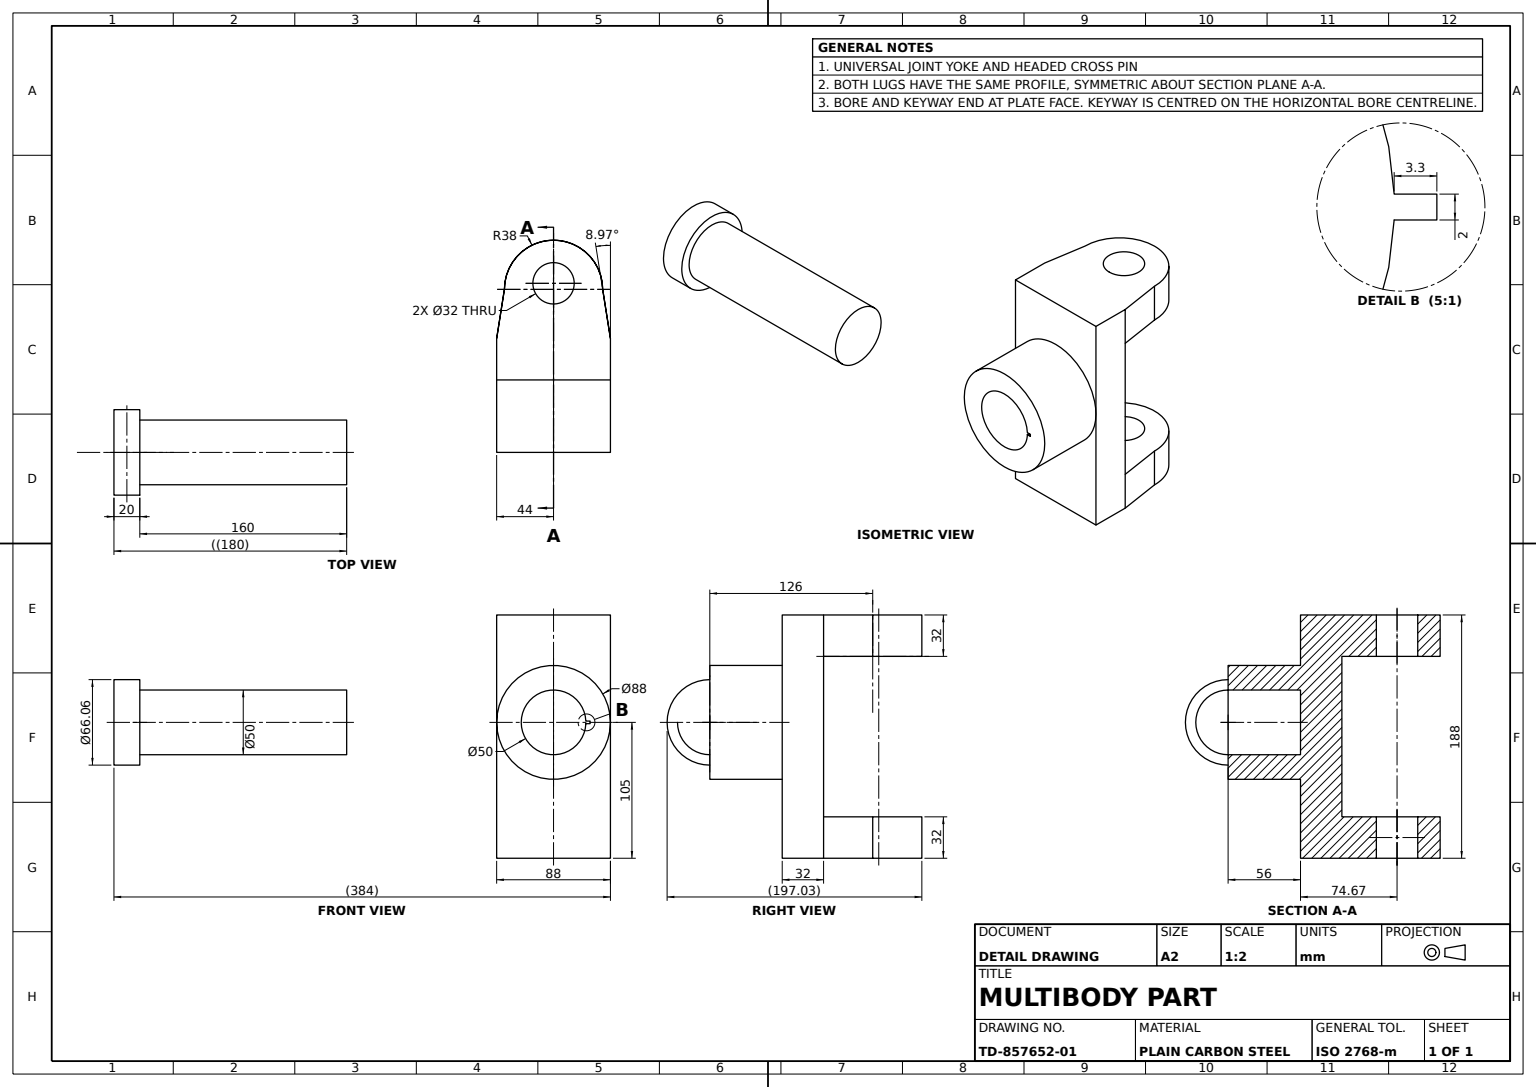
SolidWorks part; units mm, degrees
material "Plain Carbon Steel"
ref_plane "Front Plane" through (0, 0, 0) normal (0, 0, 1) x (1, 0, 0)
ref_plane "Top Plane" through (0, 0, 0) normal (0, 1, 0) x (1, 0, 0)
ref_plane "Right Plane" through (0, 0, 0) normal (1, 0, 0) x (0, 0, -1)
sketch "Hub Profile Ø88" plane through (0, 0, 0) normal (0, 0, 1) x (1, 0, 0)
  circle A0 centre (0, 0) radius 44
  dimension "D1" = 88
extrude "Hub Boss Ø88" add sketch "Hub Profile Ø88" along normal blind 56
sketch "Hub Cut Profile" plane through (0, 0, 0) normal (0, 0, -1) x (-1, 0, 0)
  line L1 (24.98, -0.9998) -> (24.98, -1.0002)
  line L2 (24.98, -1.0002) -> (28.2828, -1.0002)
  line L3 (28.2828, -1.0002) -> (28.2828, 0.9998)
  line L4 (28.2828, 0.9998) -> (24.98, 0.9998)
  arc A0 (24.98, 0.9998) -> (24.98, -0.9998) centre (0, 0) ccw
  circle A1 centre (0, 0) radius 44 construction
  dimension "D1" = 25
  dimension "D2" = 24.98
  dimension "D3" = 28.2828
  dimension "D4" = 1.0002
extrude "Hub Cut" cut sketch "Hub Cut Profile" against normal blind 56
sketch "Yoke Base Profile" plane through (0, 0, 56) normal (0, 0, 1) x (1, 0, 0)
  line L0 (-44, 0) -> (-44, 83)
  line L1 (-44, 83) -> (44, 83)
  line L2 (44, 83) -> (44, -105)
  line L3 (44, -105) -> (-44, -105)
  line L4 (-44, -105) -> (-44, 0)
  line L5 (-24.98, -0.9998) -> (-24.98, -1.0002) construction
  line L6 (-24.98, -1.0002) -> (-28.2828, -1.0002) construction
  circle A0 centre (0, 0) radius 44 construction
  dimension "D1" = 68.98
  dimension "D2" = 19.02
  dimension "D3" = 84.0002
  dimension "D4" = 103.9998
extrude "Yoke Base Plate" add sketch "Yoke Base Profile" along normal blind 32
sketch "Yoke Arms Profile" plane through (0, 83, 0) normal (0, 1, 0) x (1, 0, 0)
  line L0 (-44, -88) -> (44, -88)
  line L2 (44, -88) -> (38, -126)
  line L3 (-44, -88) -> (-38, -126)
  arc A0 (-38, -126) -> (38, -126) centre (0, -126) ccw
  dimension "D3" = 38
  dimension "D1" = 88
  dimension "D2" = 38
  dimension "D4" = 126
extrude "Yoke Arms" add sketch "Yoke Arms Profile" against normal blind 32
sketch "Yoke Web Profile" plane through (0, -105, 0) normal (0, -1, 0) x (1, 0, 0)
  line L3 (-38, 126) -> (-44, 88)
  line L4 (-44, 88) -> (44, 88)
  line L5 (44, 88) -> (38, 126)
  arc A0 (38, 126) -> (-38, 126) centre (0, 126) ccw
extrude "Yoke Web" add sketch "Yoke Web Profile" against normal blind 32
sketch "Cross Pin Bore Profile" plane through (0, 83, 0) normal (0, 1, 0) x (1, 0, 0)
  line L0 (-44, -88) -> (-44, -56) construction
  line L1 (44, -56) -> (-44, -56) construction
  circle A0 centre (0, -130.6675) radius 16
  dimension "D1" = 32
  dimension "D2" = 44
  dimension "D3" = 74.6675
extrude "Cross Pin Bore Through Lugs" cut sketch "Cross Pin Bore Profile" against normal blind 698
ref_plane "Plane1" through (0, 0, -30) normal (0, 0, 1) x (1, 0, 0)
ref_plane "Plane2" through (160, 0, 0) normal (1, 0, 0) x (0, 0, -1)
sketch "Pin Shaft Profile Ø50" plane through (160, 0, 0) normal (1, 0, 0) x (0, 0, -1)
  circle A0 centre (0, 0) radius 25
  dimension "D1" = 50
extrude "Pin Shaft Ø50" add sketch "Pin Shaft Profile Ø50" along normal blind 180 separate body
sketch "Pin Head Profile" plane through (340, 0, 0) normal (1, 0, 0) x (0, 0, -1)
  circle A0 centre (0, 0) radius 33.0291
  dimension "D1" = 66.0582
extrude "Pin Head" add sketch "Pin Head Profile" against normal blind 20
ref_plane "Plane3" through (0, -290, 0) normal (0, 1, 0) x (1, 0, 0)
